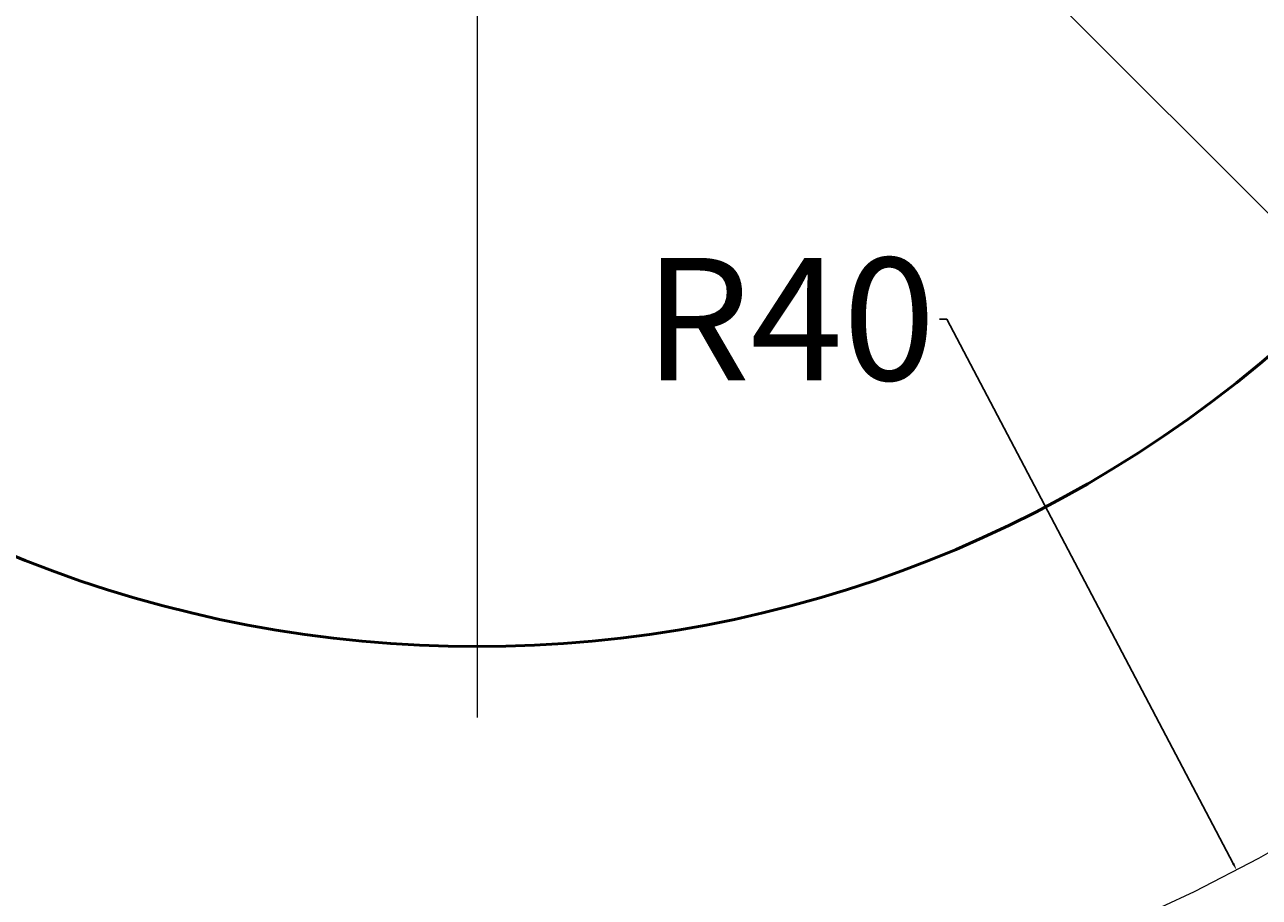
# Model space of a CAD drawing. Units: millimetres. Extents: x -53 to 92, y -147 to 37.
# Tile 5 of 16: x 8 to 38, y -90 to -69. Entities that reach past the tile are written whole.
import ezdxf

# ---------------------------------------------------------------- set-up
doc = ezdxf.new("R2010")
doc.units = ezdxf.units.MM
doc.header["$MEASUREMENT"] = 0
doc.linetypes.add('CENTER', pattern=[50.8, 31.75, -6.35, 6.35, -6.35])
for name, color, linetype, lineweight in [('M-CNTR', 4, 'CENTER', 18), ('M-DIMS', 2, 'Continuous', 25), ('M-OUTL', 7, 'Continuous', 50)]:
    doc.layers.add(name, color=color, linetype=linetype, lineweight=lineweight)
doc.styles.get("Standard").update_dxf_attribs({"font": 'arial.ttf'})
doc.dimstyles.get("Standard").update_dxf_attribs({"dimtxt": 0.18, "dimasz": 0.18, "dimexe": 0.18, "dimexo": 0.0625, "dimgap": 0.09, "dimtad": 0, "dimtih": 1, "dimtoh": 1, "dimdec": 4, "dimzin": 0, "dimdsep": 46, "dimtxsty": 'Standard', "dimcen": 0.09, "dimadec": 0, "dimazin": 0, "dimtfac": 1, "dimtdec": 4, "dimtofl": 0, "dimtmove": 0, "dimatfit": 3, "dimfxl": 1, "dimtolj": 1, "dimtzin": 0, "dimarcsym": 0})

# ---------------------------------------------------------------- blocks, each defined once
blk = doc.blocks.new('*D10')
at = {"layer": 'Defpoints', "color": 0, "transparency": 16777216}
for p in [(64.593, -18.184), (-26.68, -89.776)]:
    blk.add_point(p, dxfattribs=at)
at = {"layer": 'M-DIMS', "color": 0, "lineweight": -2, "transparency": 16777216}
for p, q in [((77.384, -8.151), (64.734, -18.073)), ((77.564, -8.151), (77.384, -8.151)), ((18.866, -53.98), (19.046, -53.98)), ((18.956, -54.07), (18.956, -53.89))]:
    blk.add_line(p, q, dxfattribs=at)
at = {"layer": 'M-DIMS', "color": 0, "transparency": 16777216}
blk.add_solid([(64.716, -18.05), (64.753, -18.097), (64.593, -18.184)], dxfattribs=at)
at = {"layer": 'M-DIMS', "color": 0, "transparency": 16777216, "insert": (82.599, -8.151), "char_height": 0.18, "attachment_point": 5}
blk.add_mtext('\\A1;{\\H16.66667x;%%C116}', dxfattribs=at)
blk = doc.blocks.new('*D12')
at = {"layer": 'Defpoints', "color": 0, "transparency": 16777216}
for p in [(18.956, -54.07), (37.579, -89.471)]:
    blk.add_point(p, dxfattribs=at)
at = {"layer": 'M-DIMS', "color": 0, "lineweight": -2, "transparency": 16777216}
for p, q in [((30.294, -75.965), (30.474, -75.965)), ((30.474, -75.965), (37.495, -89.311))]:
    blk.add_line(p, q, dxfattribs=at)
at = {"layer": 'M-DIMS', "color": 0, "transparency": 16777216}
blk.add_solid([(37.522, -89.297), (37.469, -89.325), (37.579, -89.471)], dxfattribs=at)
at = {"layer": 'M-DIMS', "color": 0, "transparency": 16777216, "insert": (26.625, -75.965), "char_height": 0.18, "attachment_point": 5}
blk.add_mtext('\\A1;{\\H16.66667x;R40}', dxfattribs=at)
blk = doc.blocks.new('*D17')
at = {"layer": 'Defpoints', "color": 0, "transparency": 16777216}
for p in [(-46.81, 25.909), (28.564, 25.909), (18.165, -111.975)]:
    blk.add_point(p, dxfattribs=at)
at = {"layer": 'M-DIMS', "color": 0, "lineweight": -2, "transparency": 16777216}
for p, q in [((28.502, 25.909), (-46.99, 25.909)), ((-46.81, 25.729), (-46.81, -42.851)), ((-46.81, -111.795), (-46.81, -43.215)), ((18.102, -111.975), (-46.99, -111.975))]:
    blk.add_line(p, q, dxfattribs=at)
at = {"layer": 'M-DIMS', "color": 0, "transparency": 16777216}
for points in [[(-46.84, 25.729), (-46.78, 25.729), (-46.81, 25.909)], [(-46.84, -111.795), (-46.78, -111.795), (-46.81, -111.975)]]:
    blk.add_solid(points, dxfattribs=at)
at = {"layer": 'M-DIMS', "color": 0, "transparency": 16777216, "insert": (-46.81, -43.033), "char_height": 0.18, "attachment_point": 5}
blk.add_mtext('\\A1;137.88', dxfattribs=at)
blk = doc.blocks.new('*D18')
at = {"layer": 'Defpoints', "color": 0, "transparency": 16777216}
for p in [(19.753, 4.014), (18.16, -111.975)]:
    blk.add_point(p, dxfattribs=at)
at = {"layer": 'M-DIMS', "color": 0, "lineweight": -2, "transparency": 16777216}
for p, q in [((18.866, -53.98), (19.046, -53.98)), ((18.956, -54.07), (18.956, -53.89)), ((17.682, -146.771), (18.158, -112.155)), ((17.502, -146.771), (17.682, -146.771))]:
    blk.add_line(p, q, dxfattribs=at)
at = {"layer": 'M-DIMS', "color": 0, "transparency": 16777216}
blk.add_solid([(18.128, -112.154), (18.188, -112.155), (18.16, -111.975)], dxfattribs=at)
at = {"layer": 'M-DIMS', "color": 0, "transparency": 16777216, "insert": (17.115, -146.771), "char_height": 0.18, "attachment_point": 5}
blk.add_mtext('\\A1;∅116', dxfattribs=at)
blk = doc.blocks.new('*D23')
at = {"layer": 'Defpoints', "color": 0, "transparency": 16777216}
for p in [(18.956, -54.07), (18.954, -94.07)]:
    blk.add_point(p, dxfattribs=at)
at = {"layer": 'M-DIMS', "color": 0, "lineweight": -2, "transparency": 16777216}
for p, q in [((18.866, -54.07), (19.046, -54.07)), ((18.956, -54.16), (18.956, -53.98)), ((18.953, -118.07), (18.954, -94.25)), ((18.773, -118.07), (18.953, -118.07))]:
    blk.add_line(p, q, dxfattribs=at)
at = {"layer": 'M-DIMS', "color": 0, "transparency": 16777216}
blk.add_solid([(18.924, -94.25), (18.984, -94.25), (18.954, -94.07)], dxfattribs=at)
at = {"layer": 'M-DIMS', "color": 0, "transparency": 16777216, "insert": (18.468, -118.07), "char_height": 0.18, "attachment_point": 5}
blk.add_mtext('\\A1;R40', dxfattribs=at)
blk = doc.blocks.new('*D24')
at = {"layer": 'Defpoints', "color": 0, "transparency": 16777216}
for p in [(18.956, -53.969), (2.002, -101.015)]:
    blk.add_point(p, dxfattribs=at)
at = {"layer": 'M-DIMS', "color": 0, "lineweight": -2, "transparency": 16777216}
for p, q in [((18.956, -54.059), (18.956, -53.879)), ((18.866, -53.969), (19.046, -53.969)), ((-8.171, -129.243), (1.941, -101.184)), ((-8.351, -129.243), (-8.171, -129.243))]:
    blk.add_line(p, q, dxfattribs=at)
at = {"layer": 'M-DIMS', "color": 0, "transparency": 16777216}
blk.add_solid([(1.912, -101.174), (1.969, -101.195), (2.002, -101.015)], dxfattribs=at)
at = {"layer": 'M-DIMS', "color": 0, "transparency": 16777216, "insert": (-8.813, -129.243), "char_height": 0.18, "attachment_point": 5}
blk.add_mtext('\\A1;R50.01', dxfattribs=at)

msp = doc.modelspace()

# ---------------------------------------------------------------- linework, layer by layer
at = {"layer": 'M-CNTR'}
for q in [(64.91832, -99.94201), (18.95638, -130.36235)]:
    msp.add_line((18.95638, -53.98007), q, dxfattribs=at)
msp.add_arc((18.95638, -54.07007), 40, 187.365915, 352.627832, dxfattribs=at)
at = {"layer": 'M-OUTL'}
for centre, radius, start, end in [((18.95638, -53.98007), 58, 108.3895553, 70.0459142), ((18.95638, -53.98007), 30.01579, 225.928942, 314.071058), ((18.95621, -53.96903), 50.00792, 225.009078, 314.99431)]:
    msp.add_arc(centre, radius, start, end, dxfattribs=at)

# ---------------------------------------------------------------- dimensions: what is measured, and where the dimension line sits
at = {"layer": 'M-DIMS'}
dim = msp.add_linear_dim(base=(-46.8103, 25.90924), p1=(18.16452, -111.97467), p2=(28.56407, 25.90924), angle=90, dimstyle='Standard', override={"dimdec": 2, "dimlfac": 1, "dimrnd": 0, "dimzin": 0, "dimdsep": 46, "dimlunit": 2}, dxfattribs=at)
dim.commit()
dim.dimension.update_dxf_attribs({"geometry": '*D17', "text_midpoint": (-46.8103, -43.03271)})
dim = msp.add_diameter_dim_2p(p1=(19.75275, 4.01446), p2=(18.16001, -111.9746), dimstyle='Standard', override={"dimdec": 0, "dimlfac": 1, "dimrnd": 0, "dimzin": 0, "dimdsep": 46, "dimlunit": 2}, dxfattribs=at)
dim.commit()
dim.dimension.update_dxf_attribs({"geometry": '*D18', "text_midpoint": (17.11548, -146.77132), "dimtype": 163})
dim = msp.add_diameter_dim_2p(p1=(-26.67986, -89.77579), p2=(64.59262, -18.18435), text='{\\H16.66667x;%%C116}', dimstyle='Standard', override={"dimclrd": 0, "dimclre": 0, "dimclrt": 0}, dxfattribs=at)
dim.commit()
dim.dimension.update_dxf_attribs({"geometry": '*D10', "text_midpoint": (82.59889, -8.15132), "dimtype": 163})
for center, mpoint, override, picture, middle in [((18.95621, -53.96903), (2.00175, -101.01516), {"dimdec": 2, "dimlfac": 1, "dimrnd": 0, "dimzin": 0, "dimdsep": 46, "dimlunit": 2}, '*D24', (-8.8134, -129.24283)), ((18.95638, -54.07007), (18.954, -94.07007), {"dimdec": 0, "dimlfac": 1, "dimrnd": 0, "dimzin": 0, "dimdsep": 46, "dimlunit": 2}, '*D23', (18.46782, -118.07007))]:
    dim = msp.add_radius_dim(center=center, mpoint=mpoint, dimstyle='Standard', override=override, dxfattribs=at)
    dim.commit()
    dim.dimension.update_dxf_attribs({"geometry": picture, "text_midpoint": middle, "dimtype": 164})
dim = msp.add_radius_dim(center=(18.95638, -54.07007), mpoint=(37.5792, -89.4705), text='{\\H16.66667x;R40}', dimstyle='Standard', override={"dimclrd": 0, "dimclre": 0, "dimclrt": 0}, dxfattribs=at)
dim.commit()
dim.dimension.update_dxf_attribs({"geometry": '*D12', "text_midpoint": (26.62522, -75.96478), "dimtype": 164})

doc.saveas('drawing.dxf')
